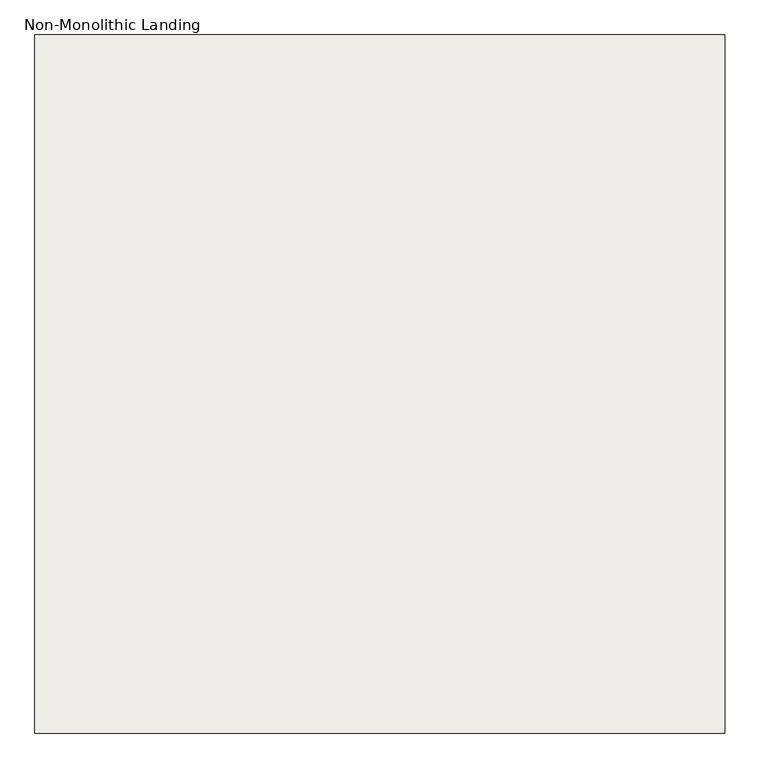
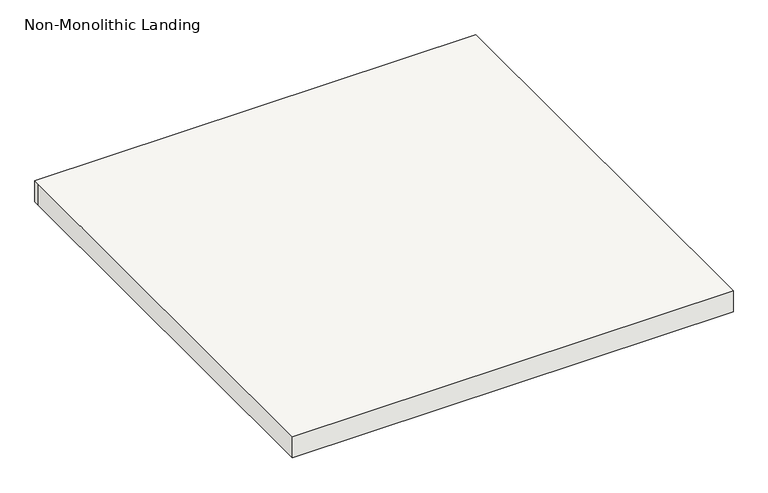
"""IFC4 building model written with IfcOpenShell, lengths in millimetres: slab geometry, Non-Monolithic Landing."""

from ifc_helpers import new_model, si_unit, frame, origin, place, context, project, spatial, polyline, outline, extrude, source, transform, mapped, element, save


def non_monolithic_landing_0691aa35(model_context):
    return source(origin(), model_context, "Body", "SweptSolid", [
        extrude(outline(polyline([(-9477.5794909, -3248.5618509), (-9477.5794909, -4251.1618509), (-10468.1794909, -4251.1618509), (-10468.1794909, -3260.5618509), (-10468.1794909, -3248.5618509), (-9477.5794909, -3248.5618509)])), frame((0.0, 0.0, 2020.8470588), z_axis=(0.0, 0.0, 1.0), x_axis=(1.0, 0.0, 0.0)), (0.0, 0.0, 1.0), 50.0),
    ])


if __name__ == "__main__":
    model = new_model("IFC4")
    model_context = context("Model", 3, world=origin())
    ifc_project = project(units=[si_unit("LENGTHUNIT", "METRE", prefix="MILLI")], contexts=[model_context])
    site = spatial("IfcSite", under=ifc_project)
    building = spatial("IfcBuilding", under=site)
    placement = place(None, origin())
    non_monolithic_landing_shape = non_monolithic_landing_0691aa35(model_context)
    element("IfcSlab", 1, ObjectType="Non-Monolithic Landing", at=placement, inside=building, context=model_context, shape_type="MappedRepresentation", body=[
        mapped(non_monolithic_landing_shape, transform((0.0, 0.0, 0.0), x_axis=(1.0, 0.0, 0.0), y_axis=(0.0, 1.0, 0.0), z_axis=(0.0, 0.0, 1.0))),
    ])
    save(model, "model.ifc")
